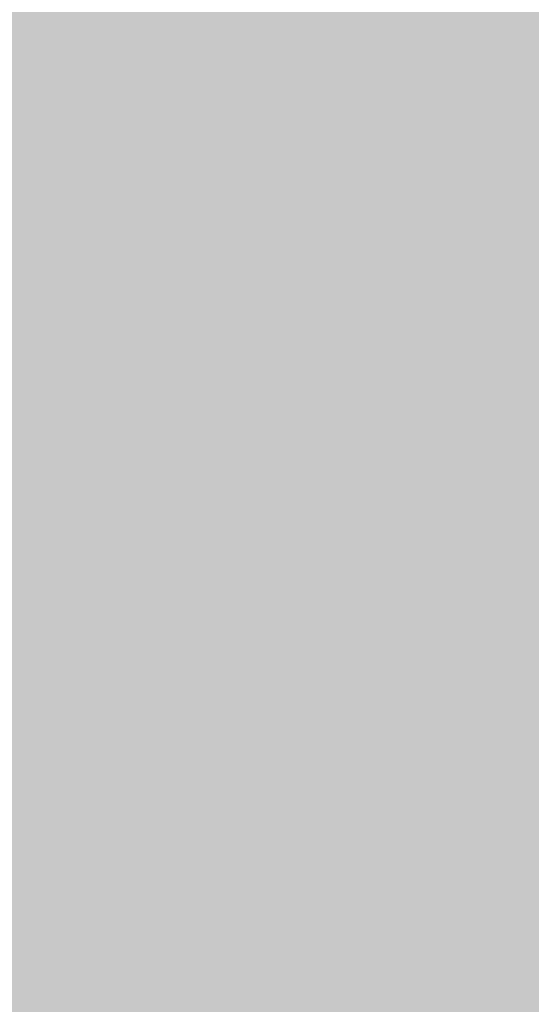
# Model space of a CAD drawing. Units: inches. Extents: x 2083 to 3317, y 1141 to 2115.
# Tile 226 of 256: x 3123.979 to 3126.132, y 1267.234 to 1271.372. Entities that reach past the tile are written whole.
import ezdxf

# ---------------------------------------------------------------- set-up
doc = ezdxf.new("R2010")
doc.units = ezdxf.units.IN
doc.layers.add('A-ANNO-DIMS', color=2, linetype='Continuous', lineweight=18)
doc.layers.add('A-WALL-PATT', color=251, linetype='Continuous', lineweight=13, true_color=0x636466)
doc.styles.get("Standard").update_dxf_attribs({"font": 'arial.ttf'})
doc.dimstyles.new('ISO-25', dxfattribs={"dimtxt": 12, "dimasz": 12, "dimexe": 1.25, "dimexo": 0.625, "dimtad": 1, "dimlunit": 3, "dimtxsty": 'Standard', "dimcen": 2.5, "dimadec": 0, "dimazin": 0, "dimtfac": 1, "dimtmove": 0, "dimatfit": 3, "dimfxl": 1, "dimarcsym": 0})

# ---------------------------------------------------------------- blocks, each defined once
blk = doc.blocks.new('*D26')
at = {"layer": 'A-ANNO-DIMS', "color": 0, "lineweight": -2, "transparency": 16777216}
for p, q in [((3088.9858, 1274.9151), (3088.9858, 1270.952)), ((3111.24, 1274.9151), (3111.24, 1270.952)), ((3076.9858, 1272.202), (2840.2624, 1272.202)), ((3111.24, 1272.202), (3088.9858, 1272.202)), ((3123.24, 1272.202), (3135.24, 1272.202))]:
    blk.add_line(p, q, dxfattribs=at)
at = {"layer": 'A-ANNO-DIMS', "color": 0, "transparency": 16777216}
for points in [[(3076.9858, 1274.202), (3076.9858, 1270.202), (3088.9858, 1272.202)], [(3123.24, 1274.202), (3123.24, 1270.202), (3111.24, 1272.202)]]:
    blk.add_solid(points, dxfattribs=at)
at = {"layer": 'Defpoints', "color": 0, "transparency": 16777216}
for p in [(3088.9858, 1275.5401), (3111.24, 1275.5401), (3088.9858, 1272.202)]:
    blk.add_point(p, dxfattribs=at)
at = {"layer": 'A-ANNO-DIMS', "color": 0, "transparency": 16777216, "insert": (2952.6241, 1279.0316), "char_height": 12, "attachment_point": 5}
blk.add_mtext('NIGHTSTAND 1\'-10 1/2" TYP.', dxfattribs=at)
blk = doc.blocks.new('*D27')
at = {"layer": 'A-ANNO-DIMS', "color": 0, "lineweight": -2, "transparency": 16777216}
for p, q in [((3114.5782, 1309.7943), (3114.5782, 1321.7943)), ((3111.865, 1297.7943), (3115.8282, 1297.7943)), ((3114.5782, 1297.7943), (3114.5782, 1275.5401)), ((3111.865, 1275.5401), (3115.8282, 1275.5401)), ((3114.5782, 1263.5401), (3114.5782, 1140.9886))]:
    blk.add_line(p, q, dxfattribs=at)
at = {"layer": 'A-ANNO-DIMS', "color": 0, "transparency": 16777216}
for points in [[(3112.5782, 1309.7943), (3116.5782, 1309.7943), (3114.5782, 1297.7943)], [(3112.5782, 1263.5401), (3116.5782, 1263.5401), (3114.5782, 1275.5401)]]:
    blk.add_solid(points, dxfattribs=at)
at = {"layer": 'Defpoints', "color": 0, "transparency": 16777216}
for p in [(3111.24, 1297.7943), (3111.24, 1275.5401), (3114.5782, 1275.5401)]:
    blk.add_point(p, dxfattribs=at)
at = {"layer": 'A-ANNO-DIMS', "color": 0, "transparency": 16777216, "insert": (3107.7485, 1196.2643), "char_height": 12, "attachment_point": 5, "rotation": 90}
blk.add_mtext('1\'-10 1/2" TYP.', dxfattribs=at)

msp = doc.modelspace()

# ---------------------------------------------------------------- hatches: boundary and pattern name
at = {"layer": 'A-WALL-PATT'}
h = msp.add_hatch(color=256, dxfattribs=at)
h.dxf.hatch_style = 1
h.paths.add_polyline_path([(3126.9598, 2020.7614), (2748.9598, 2020.7614), (2604.9598, 2020.7614), (2226.9598, 2020.7614), (2226.9598, 1702.7614), (2466.9598, 1702.7614), (2466.9598, 1582.7614), (2418.9598, 1582.7614), (2418.9598, 1477.7614), (2226.9598, 1477.7614), (2226.9598, 1263.2614), (2544.9598, 1263.2614), (2544.9598, 1411.7614), (2604.9598, 1411.7614), (2685.9598, 1411.7614), (2685.9598, 1420.7614), (2604.9598, 1420.7614), (2604.9598, 1573.7614), (2604.9598, 1702.7614), (2604.9598, 2011.7614), (2748.9598, 2011.7614), (2748.9598, 1702.7614), (2862.9598, 1702.7614), (2862.9598, 1621.7614), (2871.9598, 1621.7614), (2871.9598, 1702.7614), (2883.9598, 1702.7614), (2883.9598, 1706.9395, -0.026459), (2883.9598, 1711.7614), (2757.9598, 1711.7614), (2757.9598, 1807.7614), (2787.9598, 1807.7614), (2787.9598, 1812.2614), (2757.9598, 1812.2614), (2757.9598, 2011.7614), (2877.9598, 2011.7614), (2877.9598, 1812.2614), (2847.9598, 1812.2614), (2847.9598, 1807.7614), (2889.8357, 1807.7614), (2889.8357, 1812.2614), (2882.4598, 1812.2614), (2882.4598, 2011.7614), (3117.9598, 2011.7614), (3117.9598, 1812.2614), (2937.8357, 1812.2614), (2937.8357, 1807.7614), (2995.7098, 1807.7614), (2995.7098, 1796.1177), (3000.2098, 1796.1177), (3000.2098, 1807.7614), (3117.9598, 1807.7614), (3117.9598, 1711.7614), (3000.2098, 1711.7614), (3000.2098, 1760.1177), (2998.5727, 1760.1177, -0.020711), (2995.7098, 1760.1177), (2995.7098, 1711.7614), (2931.9598, 1711.7614), (2931.9598, 1702.7614), (3126.9598, 1702.7614)])
h.paths.add_polyline_path([(2471.4598, 2011.7614), (2471.4598, 1810.0114), (2462.7169, 1810.0114), (2462.7169, 1805.5114), (2505.9598, 1805.5114), (2505.9598, 1810.0114), (2475.9598, 1810.0114), (2475.9598, 2011.7614), (2595.9598, 2011.7614), (2595.9598, 1810.0114), (2565.9598, 1810.0114), (2565.9598, 1805.5114), (2595.9598, 1805.5114), (2595.9598, 1711.7614), (2235.9598, 1711.7614), (2235.9598, 1805.5114), (2353.7098, 1805.5114), (2353.7098, 1796.0542), (2358.2098, 1796.0542), (2358.2098, 1805.5114), (2414.7169, 1805.5114), (2414.7169, 1810.0114), (2235.9598, 1810.0114), (2235.9598, 2011.7614)], flags=16)
h.paths.add_polyline_path([(2270.2047, 1994.61), (2270.2047, 1970.61), (2246.2047, 1970.61), (2246.2047, 1994.61)], flags=0)
edge = h.paths.add_edge_path(flags=0)
edge.add_ellipse((2332.0274, 1899.7982), major_axis=(-3.043, 3.043), ratio=0.168252, start_angle=-161.3322, end_angle=-156.3071, ccw=False)
edge.add_ellipse((2333.082, 1898.7435), major_axis=(-1.0546, 1.0546), ratio=0.453532, start_angle=-123.371, end_angle=-94.1591)
edge = h.paths.add_edge_path(flags=0)
edge.add_ellipse((2332.0274, 1968.8763), major_axis=(3.043, 3.043), ratio=0.168252, start_angle=18.6678, end_angle=23.6929)
edge.add_spline(control_points=[(2332.9256, 1970.6911), (2332.2268, 1970.3361), (2330.8937, 1969.6589), (2328.4131, 1970.9321), (2327.2039, 1967.7487), (2324.7096, 1969.9556), (2322.5328, 1967.0124), (2320.0128, 1971.2958), (2317.6803, 1968.1578), (2316.0405, 1967.102), (2315.4269, 1966.8096)], knot_values=[0, 0, 0, 0, 2.267059, 4.324559, 6.685584, 8.878641, 11.121502, 14.300359, 17.755284, 19.732645, 19.732645, 19.732645, 19.732645], degree=3, periodic=0)
edge.add_ellipse((2332.0274, 1968.8763), major_axis=(3.043, 3.043), ratio=0.168252, start_angle=18.6678, end_angle=23.6929, ccw=False)
edge.add_ellipse((2333.082, 1969.9309), major_axis=(1.0546, 1.0546), ratio=0.453532, start_angle=56.629, end_angle=85.8409, ccw=False)
edge = h.paths.add_edge_path(flags=0)
edge.add_spline(control_points=[(2296.4283, 1967.9879), (2293.6278, 1965.3363), (2287.7036, 1959.7271), (2299.7439, 1949.9957), (2294.5326, 1935.6685), (2290.5732, 1920.6035), (2293.3941, 1909.9737), (2296.1854, 1904.9665)], knot_values=[0.099185, 0.099185, 0.099185, 0.099185, 0.345301, 0.619822, 0.982653, 1.386093, 1.810555, 1.810555, 1.810555, 1.810555], degree=3, periodic=0)
edge.add_spline(control_points=[(2296.1854, 1904.9665), (2297.3836, 1902.6193), (2298.001, 1901.9493), (2298.553, 1901.4682)], knot_values=[0.006246, 0.006246, 0.006246, 0.006246, 0.055476, 0.055476, 0.055476, 0.055476], degree=3, periodic=0)
edge.add_spline(control_points=[(2298.553, 1901.4682), (2297.2586, 1900.9232), (2295.2253, 1900.2321), (2293.0602, 1900.6142), (2292.1014, 1900.7884), (2292.0896, 1900.7906)], knot_values=[0.312835, 0.312835, 0.312835, 0.312835, 0.40178, 0.474987, 0.475903, 0.475903, 0.475903, 0.475903], degree=3, periodic=0)
edge.add_arc((2292.7936, 1904.6641), 3.937, 215.4209, 259.6982, ccw=False)
edge.add_spline(control_points=[(2289.5853, 1902.3823), (2289.4767, 1902.5351), (2289.3685, 1902.688), (2289.2609, 1902.8412)], knot_values=[0.102872, 0.102872, 0.102872, 0.102872, 0.116896, 0.116896, 0.116896, 0.116896], degree=3, periodic=0)
edge.add_spline(control_points=[(2289.2609, 1902.8412), (2288.6866, 1902.5502), (2287.64, 1902.0199), (2285.8813, 1901.874), (2283.853, 1901.5044), (2281.72, 1899.7105), (2278.467, 1899.4929), (2276.1571, 1901.8832), (2272.259, 1899.8041), (2267.7776, 1901.8432), (2262.2439, 1900.184), (2257.4149, 1901.7821), (2254.3184, 1900.7261), (2253.1783, 1900.3373)], knot_values=[0, 0, 0, 0, 1.907977, 3.477176, 5.261074, 7.972851, 11.680248, 13.717921, 16.939592, 22.789562, 27.502503, 33.595215, 37.145618, 37.145618, 37.145618, 37.145618], degree=3, periodic=0)
edge.add_line((2253.1783, 1900.3373), (2250.2442, 1902.8412))
edge.add_line((2250.2442, 1902.8412), (2250.2442, 1965.8333))
edge.add_line((2250.2442, 1965.8333), (2253.1783, 1968.3371))
edge.add_spline(control_points=[(2253.1783, 1968.3371), (2254.3184, 1967.9483), (2257.4149, 1966.8924), (2262.2439, 1968.4904), (2267.7776, 1966.8313), (2271.5267, 1968.5372), (2273.8759, 1967.8283), (2274.2067, 1967.7276)], knot_values=[0, 0, 0, 0, 0.09018, 0.244935, 0.364644, 0.513233, 0.537855, 0.537855, 0.537855, 0.537855], degree=3, periodic=0)
edge.add_arc((2274.3529, 1963.7933), 3.937, 72.0511, 92.1279, ccw=False)
edge.add_arc((2281.2969, 1985.23), 18.5963, 252.05113, 288.56572)
edge.add_arc((2292.3167, 1956.0289), 12.6461, 71.02679, 113.77822, ccw=False)
edge = h.paths.add_edge_path(flags=0)
edge.add_spline(control_points=[(2274.8994, 1951.8562), (2275.0662, 1951.6166), (2275.2327, 1951.3766), (2275.398, 1951.1359)], knot_values=[1.409916, 1.409916, 1.409916, 1.409916, 1.43159, 1.43159, 1.43159, 1.43159], degree=3, periodic=0)
edge.add_spline(control_points=[(2275.398, 1951.1359), (2275.7921, 1950.5619), (2276.1792, 1949.9838), (2276.5455, 1949.3971)], knot_values=[1.358238, 1.358238, 1.358238, 1.358238, 1.409916, 1.409916, 1.409916, 1.409916], degree=3, periodic=0)
edge.add_line((2276.5455, 1949.3971), (2277.4373, 1947.8622))
edge.add_spline(control_points=[(2277.4373, 1947.8622), (2276.3038, 1945.6731), (2274.6397, 1942.4269), (2274.6316, 1938.0939), (2272.7991, 1930.8515), (2274.3564, 1943.897), (2275.9477, 1947.9234), (2276.5455, 1949.3971)], knot_values=[0.005632, 0.005632, 0.005632, 0.005632, 0.186014, 0.266002, 0.357087, 0.59639, 0.739732, 0.739732, 0.739732, 0.739732], degree=3, periodic=0)
edge.add_spline(control_points=[(2276.5455, 1949.3971), (2276.1792, 1949.9838), (2275.7921, 1950.5619), (2275.398, 1951.1359)], knot_values=[1.358238, 1.358238, 1.358238, 1.358238, 1.409916, 1.409916, 1.409916, 1.409916], degree=3, periodic=0)
edge.add_spline(control_points=[(2275.398, 1951.1359), (2274.9425, 1950.0805), (2274.2078, 1948.0253), (2273.9346, 1944.8515), (2272.4685, 1937.6275), (2273.4662, 1945.6965), (2274.7006, 1951.0595), (2274.8994, 1951.8562)], knot_values=[0.104364, 0.104364, 0.104364, 0.104364, 0.189636, 0.269624, 0.36071, 0.600013, 0.644622, 0.644622, 0.644622, 0.644622], degree=3, periodic=0)
h.paths.add_polyline_path([(2269.1675, 1963.1276, -0.357527), (2268.1706, 1960.9764, -0.092561), (2268.1706, 1939.4363, -0.357527), (2269.1675, 1937.2851, -0.357527), (2267.0163, 1938.282, -0.164785), (2254.6856, 1938.282, -0.357527), (2252.5344, 1937.2851, -0.357527), (2253.5313, 1939.4363, -0.092561), (2253.5313, 1960.9764, -0.357527), (2252.5344, 1963.1276, -0.357527), (2254.6856, 1962.1307, -0.164785), (2267.0163, 1962.1307, -0.357527)], flags=0)
h.paths.add_polyline_path([(2248.8741, 1967.8018), (2248.8741, 1957.0277), (2249.4578, 1957.0277), (2249.4578, 1911.6468), (2248.8741, 1911.6468), (2248.8741, 1900.8727), (2246.5119, 1900.8727, 0.197327), (2244.1497, 1902.4569), (2244.1497, 1966.2176, 0.197327), (2246.5119, 1967.8018)], flags=0)
h.paths.add_polyline_path([(2269.1675, 1931.3893, -0.357527), (2268.1706, 1929.2381, -0.092561), (2268.1706, 1907.6981, -0.357527), (2269.1675, 1905.5469, -0.357527), (2267.0163, 1906.5438, -0.164785), (2254.6856, 1906.5438, -0.357527), (2252.5344, 1905.5469, -0.357527), (2253.5313, 1907.6981, -0.092561), (2253.5313, 1929.2381, -0.357527), (2252.5344, 1931.3893, -0.357527), (2254.6856, 1930.3925, -0.164785), (2267.0163, 1930.3925, -0.357527)], flags=0)
edge = h.paths.add_edge_path(flags=0)
edge.add_spline(control_points=[(2276.1969, 1906.7237), (2276.1681, 1909.0289), (2276.114, 1913.3719), (2270.5984, 1924.925), (2273.9052, 1919.0128), (2275.9217, 1916.2621), (2275.4746, 1912.4021), (2277.2579, 1910.3806), (2276.696, 1908.225), (2276.6462, 1906.813), (2276.6178, 1906.0084)], knot_values=[0, 0, 0, 0, 8.61026, 16.221274, 18.843057, 23.804898, 27.440828, 29.356102, 31.203478, 33.650687, 33.650687, 33.650687, 33.650687], degree=3, periodic=0)
edge.add_spline(control_points=[(2276.6178, 1906.0084), (2276.6233, 1905.6241), (2276.4977, 1904.6287), (2275.4418, 1903.8547), (2274.9373, 1903.0804), (2274.8591, 1902.8412)], knot_values=[0.156488, 0.156488, 0.156488, 0.156488, 0.184398, 0.231376, 0.250598, 0.250598, 0.250598, 0.250598], degree=3, periodic=0)
edge.add_line((2274.8591, 1902.8412), (2276.506, 1902.8412))
edge.add_spline(control_points=[(2276.506, 1902.8412), (2276.7883, 1903.0849), (2277.6651, 1904.1252), (2278.2495, 1904.3407), (2277.6539, 1908.5274), (2278.1557, 1906.2278), (2278.1005, 1905.2859), (2278.8467, 1904.069), (2277.8568, 1903.4149), (2277.8742, 1902.991), (2277.9036, 1902.8412)], knot_values=[0.059574, 0.059574, 0.059574, 0.059574, 0.080753, 0.103741, 0.16972, 0.176036, 0.207137, 0.240474, 0.262341, 0.27366, 0.27366, 0.27366, 0.27366], degree=3, periodic=0)
edge.add_line((2277.9036, 1902.8412), (2280.0298, 1902.8412))
edge.add_spline(control_points=[(2280.0298, 1902.8412), (2279.8882, 1903.0884), (2279.4993, 1903.9816), (2280.1523, 1905.9393), (2278.1036, 1909.6578), (2279.7624, 1907.1853), (2280.3279, 1904.8749), (2280.4851, 1903.4896), (2281.4633, 1903.2494), (2281.7583, 1902.9365), (2281.834, 1902.8412)], knot_values=[0.013856, 0.013856, 0.013856, 0.013856, 0.034874, 0.088867, 0.107879, 0.126738, 0.158714, 0.193757, 0.217487, 0.226722, 0.226722, 0.226722, 0.226722], degree=3, periodic=0)
edge.add_spline(control_points=[(2281.834, 1902.8412), (2281.7875, 1902.8267), (2281.647, 1902.783), (2281.3955, 1902.8595), (2281.0881, 1902.9852), (2280.7207, 1903.0609), (2280.3335, 1903.0257), (2280.1248, 1902.8989), (2280.0298, 1902.8412)], knot_values=[0, 0, 0, 0, 0.14413, 0.435517, 0.749276, 1.153046, 1.548371, 1.878348, 1.878348, 1.878348, 1.878348], degree=3, periodic=0)
edge.add_line((2280.0298, 1902.8412), (2277.9036, 1902.8412))
edge.add_spline(control_points=[(2277.9036, 1902.8412), (2277.8929, 1902.7959), (2277.8654, 1902.6796), (2277.6075, 1902.6875), (2277.2741, 1902.8007), (2276.8379, 1902.6198), (2276.5838, 1902.7893), (2276.506, 1902.8412)], knot_values=[0, 0, 0, 0, 0.127189, 0.326199, 0.628009, 1.24357, 1.515331, 1.515331, 1.515331, 1.515331], degree=3, periodic=0)
edge.add_line((2276.506, 1902.8412), (2274.8591, 1902.8412))
edge.add_spline(control_points=[(2274.8591, 1902.8412), (2274.8144, 1902.8986), (2274.7251, 1903.0134), (2274.4935, 1903.119), (2274.2443, 1902.9605), (2273.9371, 1903.1849), (2273.614, 1902.9831), (2273.4083, 1902.883), (2273.3223, 1902.8412)], knot_values=[0, 0, 0, 0, 0.21843, 0.436957, 0.687977, 0.990379, 1.398396, 1.69185, 1.69185, 1.69185, 1.69185], degree=3, periodic=0)
edge.add_spline(control_points=[(2273.3223, 1902.8412), (2273.6167, 1903.4457), (2274.274, 1904.5383), (2276.0272, 1904.5737), (2276.207, 1906.5836), (2276.1969, 1906.7237)], knot_values=[0.012227, 0.012227, 0.012227, 0.012227, 0.059472, 0.106218, 0.134458, 0.134458, 0.134458, 0.134458], degree=3, periodic=0)
h.paths.add_polyline_path([(2270.7761, 1897.7898), (2270.7761, 1873.7898), (2246.7761, 1873.7898), (2246.7761, 1897.7898)], flags=0)
h.paths.add_polyline_path([(2353.7098, 1760.0051), (2353.7098, 1760.0542), (2358.2098, 1760.0542, -0.033729)], flags=0)
h.paths.add_polyline_path([(2321.8191, 1737.5292), (2341.9953, 1737.5292, -0.414214), (2343.2033, 1736.3212), (2343.2033, 1721.0206, -0.414214), (2341.9953, 1719.8127), (2321.8191, 1719.8127, -0.414214), (2320.6112, 1721.0206), (2320.6112, 1736.3212, -0.414214)], flags=0)
h.paths.add_polyline_path([(2324.235, 1736.3212), (2339.5794, 1736.3212, -0.414214), (2341.9953, 1733.9053), (2341.9953, 1725.4497, -0.414214), (2339.5794, 1723.0338), (2333.6806, 1723.0338), (2333.8453, 1722.0455, -0.870646), (2335.4254, 1721.8259, -0.767327), (2333.9227, 1721.4232), (2331.291, 1721.4232, -0.767327), (2329.7883, 1721.8259, -0.870646), (2331.3684, 1722.0455), (2331.5331, 1723.0338), (2324.235, 1723.0338, -0.414214), (2321.8191, 1725.4497), (2321.8191, 1733.9053, -0.414214)], flags=0)
h.paths.add_polyline_path([(2570.4838, 1928.6154), (2589.6838, 1928.6154), (2590.1688, 1928.6154), (2590.1688, 1904.9934), (2570.4838, 1904.9934)], flags=0)
h.paths.add_polyline_path([(2574.4473, 1927.2638, -1), (2572.8288, 1927.2638, -1)], flags=0)
h.paths.add_polyline_path([(2573.0899, 1926.9409), (2573.925, 1927.776), (2574.1477, 1927.5533), (2573.3126, 1926.7182)], flags=0)
h.paths.add_polyline_path([(2578.7791, 1919.7296, -1), (2571.5917, 1919.7296, -1)], flags=0)
h.paths.add_polyline_path([(2578.3854, 1919.7296, -1), (2571.9854, 1919.7296, -1)], flags=0)
h.paths.add_polyline_path([(2331.5958, 1729.4762, -1), (2333.618, 1729.4762, -1)], flags=0)
h.paths.add_polyline_path([(2578.0342, 1927.2638, -1), (2576.4157, 1927.2638, -1)], flags=0)
h.paths.add_polyline_path([(2576.6889, 1927.5311), (2576.9116, 1927.7538), (2577.7467, 1926.9186), (2577.524, 1926.6959)], flags=0)
h.paths.add_polyline_path([(2578.1391, 1909.8595, -1), (2572.2317, 1909.8595, -1)], flags=0)
h.paths.add_polyline_path([(2577.7454, 1909.8595, -1), (2572.6254, 1909.8595, -1)], flags=0)
h.paths.add_polyline_path([(2583.7977, 1927.2638, -1), (2582.1792, 1927.2638, -1)], flags=0)
h.paths.add_polyline_path([(2582.7186, 1927.7538), (2583.5538, 1926.9186), (2583.3311, 1926.6959), (2582.4959, 1927.5311)], flags=0)
h.paths.add_polyline_path([(2582.4959, 1927.5311), (2582.7186, 1927.7538), (2583.5538, 1926.9186), (2583.3311, 1926.6959)], flags=0)
h.paths.add_polyline_path([(2587.7391, 1920.5296, -1), (2581.8317, 1920.5296, -1)], flags=0)
h.paths.add_polyline_path([(2587.3454, 1920.5296, -1), (2582.2254, 1920.5296, -1)], flags=0)
h.paths.add_polyline_path([(2587.3846, 1927.2638, -1), (2585.7661, 1927.2638, -1)], flags=0)
h.paths.add_polyline_path([(2586.082, 1926.9802), (2586.9172, 1927.8154), (2587.1399, 1927.5927), (2586.3047, 1926.7575)], flags=0)
h.paths.add_polyline_path([(2588.3791, 1910.6595, -1), (2581.1917, 1910.6595, -1)], flags=0)
h.paths.add_polyline_path([(2587.9854, 1910.6595, -1), (2581.5854, 1910.6595, -1)], flags=0)
h.paths.add_polyline_path([(2417.1677, 1729.4779), (2437.3439, 1729.4779, -0.414214), (2438.5519, 1728.2699), (2438.5519, 1712.9693, -0.414214), (2437.3439, 1711.7614), (2417.1677, 1711.7614, -0.414214), (2415.9598, 1712.9693), (2415.9598, 1728.2699, -0.414214)], flags=0)
h.paths.add_polyline_path([(2419.5836, 1728.2699), (2434.928, 1728.2699, -0.414214), (2437.3439, 1725.8541), (2437.3439, 1717.3984, -0.414214), (2434.928, 1714.9825), (2429.0292, 1714.9825), (2429.1939, 1713.9942, -0.870646), (2430.774, 1713.7746, -0.767327), (2429.2713, 1713.372), (2426.6396, 1713.372, -0.767327), (2425.1369, 1713.7746, -0.870646), (2426.717, 1713.9942), (2426.8817, 1714.9825), (2419.5836, 1714.9825, -0.414214), (2417.1677, 1717.3984), (2417.1677, 1725.8541, -0.414214)], flags=0)
h.paths.add_polyline_path([(2419.5836, 1728.2699), (2434.928, 1728.2699, -0.414214), (2437.3439, 1725.8541), (2437.3439, 1717.3984, -0.414214), (2434.928, 1714.9825), (2429.0292, 1714.9825), (2428.3581, 1719.009), (2427.5528, 1719.009), (2426.8817, 1714.9825), (2419.5836, 1714.9825, -0.414214), (2417.1677, 1717.3984), (2417.1677, 1725.8541, -0.414214)], flags=0)
h.paths.add_polyline_path([(2426.9444, 1721.4249, -1), (2428.9666, 1721.4249, -1)], flags=0)
h.paths.add_polyline_path([(2475.9598, 1702.7614), (2595.9598, 1702.7614), (2595.9598, 1582.7614), (2475.9598, 1582.7614)], flags=16)
h.paths.add_polyline_path([(2427.9598, 1573.7614), (2595.9598, 1573.7614), (2595.9598, 1468.7614), (2595.9598, 1420.7614), (2384.4598, 1420.7614), (2384.4598, 1468.7614), (2427.9598, 1468.7614)], flags=16)
h.paths.add_polyline_path([(2379.9598, 1468.7614), (2379.9598, 1420.7614), (2235.9598, 1420.7614), (2235.9598, 1468.7614)], flags=16)
h.paths.add_polyline_path([(2317.816, 1466.6958), (2337.9922, 1466.6958, -0.414214), (2339.2002, 1465.4878), (2339.2002, 1450.1872, -0.414214), (2337.9922, 1448.9792), (2317.816, 1448.9792, -0.414214), (2316.6081, 1450.1872), (2316.6081, 1465.4878, -0.414214)], flags=0)
h.paths.add_polyline_path([(2320.2319, 1465.4878), (2335.5763, 1465.4878, -0.414214), (2337.9922, 1463.0719), (2337.9922, 1454.6163, -0.414214), (2335.5763, 1452.2004), (2329.6775, 1452.2004), (2329.8422, 1451.212, -0.870646), (2331.4223, 1450.9925, -0.767327), (2329.9196, 1450.5898), (2327.2879, 1450.5898, -0.767327), (2325.7852, 1450.9925, -0.870646), (2327.3653, 1451.212), (2327.53, 1452.2004), (2320.2319, 1452.2004, -0.414214), (2317.816, 1454.6163), (2317.816, 1463.0719, -0.414214)], flags=0)
h.paths.add_polyline_path([(2320.2319, 1465.4878), (2335.5763, 1465.4878, -0.414214), (2337.9922, 1463.0719), (2337.9922, 1454.6163, -0.414214), (2335.5763, 1452.2004), (2329.6775, 1452.2004), (2329.0064, 1456.2269), (2328.2011, 1456.2269), (2327.53, 1452.2004), (2320.2319, 1452.2004, -0.414214), (2317.816, 1454.6163), (2317.816, 1463.0719, -0.414214)], flags=0)
h.paths.add_polyline_path([(2327.5926, 1458.6428, -1), (2329.6148, 1458.6428, -1)], flags=0)
h.paths.add_polyline_path([(2244.4117, 1433.3405), (2241.9209, 1433.3405, -0.414214), (2240.0179, 1435.2435), (2240.0179, 1440.9528, -0.414211), (2241.9209, 1442.8559), (2244.4117, 1442.8559, -1.976472)], flags=0)
h.paths.add_polyline_path([(2245.3569, 1434.3975, -0.414214), (2245.3569, 1441.7988, -2.144098)], flags=0)
h.paths.add_polyline_path([(2535.9598, 1416.2614), (2535.9598, 1272.2614), (2235.9598, 1272.2614), (2235.9598, 1416.2614)], flags=16)
h.paths.add_polyline_path([(2260.1196, 1384.2928), (2260.1196, 1362.0386), (2237.8654, 1362.0386), (2237.8654, 1384.2928)], flags=0)
edge = h.paths.add_edge_path(flags=0)
edge.add_line((2318.2518, 1362.0933), (2318.1458, 1362.001))
edge.add_ellipse((2317.4451, 1360.431), major_axis=(2.8216, 2.8216), ratio=0.168252, start_angle=18.6678, end_angle=20.9481, ccw=False)
edge.add_ellipse((2318.423, 1361.409), major_axis=(0.9779, 0.9779), ratio=0.453532, start_angle=56.629, end_angle=70.2262, ccw=False)
edge = h.paths.add_edge_path(flags=0)
edge.add_line((2319.1074, 1295.5711), (2319.015, 1295.6771))
edge.add_ellipse((2317.4451, 1296.3778), major_axis=(-2.8216, 2.8216), ratio=0.168252, start_angle=-161.3322, end_angle=-159.0519, ccw=False)
edge.add_ellipse((2318.423, 1295.3999), major_axis=(-0.9779, 0.9779), ratio=0.453532, start_angle=-123.371, end_angle=-109.7738)
edge = h.paths.add_edge_path(flags=0)
edge.add_spline(control_points=[(2284.2103, 1301.1702), (2284.5807, 1300.4447), (2284.8912, 1299.892), (2285.1596, 1299.461)], knot_values=[0.039066, 0.039066, 0.039066, 0.039066, 0.055476, 0.055476, 0.055476, 0.055476], degree=3, periodic=0)
edge.add_line((2285.1596, 1299.461), (2284.2103, 1301.1702))
edge = h.paths.add_edge_path(flags=0)
edge.add_line((2280.4125, 1297.298), (2283.37, 1297.0361))
edge.add_line((2283.37, 1297.0361), (2286.4057, 1297.9263))
edge.add_spline(control_points=[(2286.4057, 1297.9263), (2285.3055, 1297.4631), (2284.3448, 1297.1292), (2283.37, 1297.0361)], knot_values=[0.394369, 0.394369, 0.394369, 0.394369, 0.475903, 0.475903, 0.475903, 0.475903], degree=3, periodic=0)
edge.add_spline(control_points=[(2283.37, 1297.0361), (2283.2814, 1297.0277), (2282.3163, 1296.9573), (2281.3125, 1297.1345), (2280.4234, 1297.296), (2280.4125, 1297.298)], knot_values=[0.312835, 0.312835, 0.312835, 0.312835, 0.320246, 0.393453, 0.394369, 0.394369, 0.394369, 0.394369], degree=3, periodic=0)
edge = h.paths.add_edge_path(flags=0)
edge.add_line((2284.4356, 1359.6073), (2280.4463, 1355.328))
edge.add_line((2280.4463, 1355.328), (2279.58, 1351.0178))
edge.add_line((2279.58, 1351.0178), (2282.413, 1346.5804))
edge.add_spline(control_points=[(2282.413, 1346.5804), (2283.1533, 1345.5892), (2284.2529, 1344.0289), (2284.801, 1342.3872), (2284.9352, 1341.8055)], knot_values=[1.240098, 1.240098, 1.240098, 1.240098, 1.332892, 1.382712, 1.382712, 1.382712, 1.382712], degree=3, periodic=0)
edge.add_spline(control_points=[(2284.9352, 1341.8055), (2285.3191, 1340.1406), (2285.233, 1338.4092), (2284.9099, 1336.6541)], knot_values=[1.097484, 1.097484, 1.097484, 1.097484, 1.240098, 1.240098, 1.240098, 1.240098], degree=3, periodic=0)
edge.add_spline(control_points=[(2284.9099, 1336.6541), (2284.5868, 1334.899), (2284.0267, 1333.1203), (2283.4626, 1331.3606)], knot_values=[0.95487, 0.95487, 0.95487, 0.95487, 1.097484, 1.097484, 1.097484, 1.097484], degree=3, periodic=0)
edge.add_line((2283.4626, 1331.3606), (2281.8904, 1326.1534))
edge.add_line((2281.8904, 1326.1534), (2280.7563, 1321.0561))
edge.add_line((2280.7563, 1321.0561), (2280.2992, 1316.002))
edge.add_line((2280.2992, 1316.002), (2280.7159, 1310.9501))
edge.add_line((2280.7159, 1310.9501), (2282.0281, 1305.9721))
edge.add_line((2282.0281, 1305.9721), (2284.2103, 1301.1702))
edge.add_spline(control_points=[(2284.2103, 1301.1702), (2283.3407, 1302.7302), (2282.6119, 1304.3365), (2282.0281, 1305.9721)], knot_values=[0.099185, 0.099185, 0.099185, 0.099185, 0.241799, 0.241799, 0.241799, 0.241799], degree=3, periodic=0)
edge.add_spline(control_points=[(2282.0281, 1305.9721), (2281.4443, 1307.6078), (2281.0055, 1309.2728), (2280.7159, 1310.9501)], knot_values=[0.241799, 0.241799, 0.241799, 0.241799, 0.384413, 0.384413, 0.384413, 0.384413], degree=3, periodic=0)
edge.add_spline(control_points=[(2280.7159, 1310.9501), (2280.4332, 1312.5876), (2280.2894, 1314.277), (2280.2989, 1315.962), (2280.2992, 1316.002)], knot_values=[0.384413, 0.384413, 0.384413, 0.384413, 0.523647, 0.527028, 0.527028, 0.527028, 0.527028], degree=3, periodic=0)
edge.add_spline(control_points=[(2280.2992, 1316.002), (2280.3123, 1317.687), (2280.4779, 1319.3679), (2280.7563, 1321.0561)], knot_values=[0.527028, 0.527028, 0.527028, 0.527028, 0.669642, 0.669642, 0.669642, 0.669642], degree=3, periodic=0)
edge.add_spline(control_points=[(2280.7563, 1321.0561), (2281.0346, 1322.7443), (2281.4259, 1324.4396), (2281.8904, 1326.1534)], knot_values=[0.669642, 0.669642, 0.669642, 0.669642, 0.812256, 0.812256, 0.812256, 0.812256], degree=3, periodic=0)
edge.add_spline(control_points=[(2281.8904, 1326.1534), (2282.2644, 1327.5333), (2282.7879, 1329.2618), (2283.3528, 1331.0178), (2283.4626, 1331.3606)], knot_values=[0.812256, 0.812256, 0.812256, 0.812256, 0.927087, 0.95487, 0.95487, 0.95487, 0.95487], degree=3, periodic=0)
edge.add_line((2283.4626, 1331.3606), (2284.9099, 1336.6541))
edge.add_line((2284.9099, 1336.6541), (2284.9352, 1341.8055))
edge.add_line((2284.9352, 1341.8055), (2282.413, 1346.5804))
edge.add_spline(control_points=[(2282.413, 1346.5804), (2281.2751, 1348.1038), (2280.0784, 1349.5703), (2279.58, 1351.0178)], knot_values=[1.382712, 1.382712, 1.382712, 1.382712, 1.525326, 1.525326, 1.525326, 1.525326], degree=3, periodic=0)
edge.add_spline(control_points=[(2279.58, 1351.0178), (2279.4433, 1351.4147), (2279.1363, 1352.8569), (2279.7352, 1354.2904), (2280.4463, 1355.328)], knot_values=[1.525326, 1.525326, 1.525326, 1.525326, 1.564439, 1.667941, 1.667941, 1.667941, 1.667941], degree=3, periodic=0)
edge.add_spline(control_points=[(2280.4463, 1355.328), (2281.4261, 1356.7578), (2282.9308, 1358.1826), (2284.4356, 1359.6073)], knot_values=[1.667941, 1.667941, 1.667941, 1.667941, 1.810555, 1.810555, 1.810555, 1.810555], degree=3, periodic=0)
edge.add_arc((2280.6231, 1348.5182), 11.7262, 71.02679, 113.77822)
edge.add_arc((2270.4049, 1375.5952), 17.2436, 252.05113, 288.56572, ccw=False)
edge.add_arc((2263.966, 1355.7178), 3.6506, 72.0511, 92.1279)
edge.add_arc((2263.966, 1355.7178), 3.6506, 92.1279, 177.9851)
edge.add_spline(control_points=[(2260.3176, 1355.8462), (2260.2604, 1354.2207), (2260.5513, 1350.1865), (2262.9993, 1346.7663), (2264.4727, 1344.649)], knot_values=[1.43159, 1.43159, 1.43159, 1.43159, 1.564144, 1.770695, 1.770695, 1.770695, 1.770695], degree=3, periodic=0)
edge.add_line((2264.4727, 1344.649), (2264.9356, 1343.9825))
edge.add_spline(control_points=[(2263.801, 1340.2481), (2263.8432, 1340.5141), (2264.0672, 1341.7565), (2264.5127, 1343.0025), (2264.935, 1343.9811)], knot_values=[0.53657, 0.53657, 0.53657, 0.53657, 0.559349, 0.644622, 0.644622, 0.644622, 0.644622], degree=3, periodic=0)
edge.add_spline(control_points=[(2264.935, 1343.9811), (2265.1178, 1343.715), (2265.2989, 1343.4479), (2265.4768, 1343.1794)], knot_values=[1.384077, 1.384077, 1.384077, 1.384077, 1.409916, 1.409916, 1.409916, 1.409916], degree=3, periodic=0)
edge.add_spline(control_points=[(2265.4768, 1343.1794), (2265.6546, 1342.9108), (2265.8293, 1342.6408), (2265.9991, 1342.3688)], knot_values=[1.358238, 1.358238, 1.358238, 1.358238, 1.384077, 1.384077, 1.384077, 1.384077], degree=3, periodic=0)
edge.add_line((2265.9991, 1342.3688), (2266.826, 1340.9455))
edge.add_spline(control_points=[(2266.826, 1340.9455), (2268.8944, 1337.0897), (2271.3982, 1325.843), (2270.5162, 1310.5686), (2275.9194, 1301.8606), (2277.7895, 1299.1994)], knot_values=[0.116896, 0.116896, 0.116896, 0.116896, 0.472987, 1.050969, 1.313793, 1.313793, 1.313793, 1.313793], degree=3, periodic=0)
edge.add_spline(control_points=[(2277.7895, 1299.1994), (2277.8394, 1299.1285), (2277.8894, 1299.0575), (2277.9396, 1298.9866)], knot_values=[0.109884, 0.109884, 0.109884, 0.109884, 0.116896, 0.116896, 0.116896, 0.116896], degree=3, periodic=0)
edge.add_line((2277.9396, 1298.9866), (2277.7888, 1299.1991))
edge.add_spline(control_points=[(2277.7888, 1299.1991), (2277.2566, 1298.9294), (2276.2864, 1298.4379), (2275.0394, 1298.3344), (2274.3833, 1298.2389), (2274.2153, 1298.2093)], knot_values=[33.12187, 33.12187, 33.12187, 33.12187, 35.029056, 36.598255, 37.144827, 37.144827, 37.144827, 37.144827], degree=3, periodic=0)
edge.add_line((2274.2153, 1298.2093), (2273.0731, 1297.893))
edge.add_spline(control_points=[(2273.0731, 1297.893), (2272.3229, 1297.5798), (2271.0392, 1296.5105), (2269.2484, 1296.2261), (2268.4231, 1296.3747)], knot_values=[26.532584, 26.532584, 26.532584, 26.532584, 29.198919, 31.839101, 31.839101, 31.839101, 31.839101], degree=3, periodic=0)
edge.add_line((2268.4231, 1296.3747), (2263.8785, 1297.4575))
edge.add_spline(control_points=[(2263.8785, 1297.4575), (2263.5561, 1297.3594), (2261.8603, 1296.8387), (2260.2388, 1297.2824), (2258.9335, 1297.5165)], knot_values=[15.919551, 15.919551, 15.919551, 15.919551, 16.939592, 21.226067, 21.226067, 21.226067, 21.226067], degree=3, periodic=0)
edge.add_line((2258.9335, 1297.5165), (2254.0552, 1297.329))
edge.add_spline(control_points=[(2254.0552, 1297.329), (2253.7555, 1297.2958), (2252.1137, 1297.1652), (2250.4619, 1297.5442), (2249.1297, 1297.6679)], knot_values=[5.306517, 5.306517, 5.306517, 5.306517, 6.276435, 10.613034, 10.613034, 10.613034, 10.613034], degree=3, periodic=0)
edge.add_line((2249.1297, 1297.6679), (2244.3316, 1296.8778))
edge.add_line((2244.3316, 1296.8778), (2241.611, 1299.1994))
edge.add_line((2241.611, 1299.1994), (2241.611, 1357.6094))
edge.add_line((2241.611, 1357.6094), (2244.3316, 1359.9311))
edge.add_line((2244.3316, 1359.9311), (2252.7288, 1359.5427))
edge.add_spline(control_points=[(2252.7288, 1359.5427), (2252.8709, 1359.5464), (2253.3057, 1359.5482), (2253.7398, 1359.5143), (2254.0317, 1359.4824)], knot_values=[0.233291, 0.233291, 0.233291, 0.233291, 0.244935, 0.268927, 0.268927, 0.268927, 0.268927], degree=3, periodic=0)
edge.add_line((2254.0317, 1359.4824), (2259.5872, 1359.4164))
edge.add_spline(control_points=[(2259.5872, 1359.4164), (2260.6771, 1359.6285), (2262.0732, 1359.897), (2263.5237, 1359.4593), (2263.8304, 1359.366)], knot_values=[0.422516, 0.422516, 0.422516, 0.422516, 0.513233, 0.537855, 0.537855, 0.537855, 0.537855], degree=3, periodic=0)
edge.add_arc((2263.966, 1355.7178), 3.6506, 72.0511, 92.1279, ccw=False)
edge.add_arc((2270.4049, 1375.5952), 17.2436, 252.05113, 288.56572)
edge.add_arc((2280.6231, 1348.5182), 11.7262, 71.02679, 113.77822, ccw=False)
h.paths.add_polyline_path([(2240.3405, 1359.4347), (2240.3405, 1349.4444), (2240.8818, 1349.4444), (2240.8818, 1307.3645), (2240.3405, 1307.3645), (2240.3405, 1297.3741), (2238.1502, 1297.3741, 0.197327), (2235.9598, 1298.8431), (2235.9598, 1357.9657, 0.197327), (2238.1502, 1359.4347)], flags=0)
h.paths.add_polyline_path([(2259.1578, 1355.1005, -0.357527), (2258.2334, 1353.1058, -0.092561), (2258.2334, 1333.1326, -0.357527), (2259.1578, 1331.1379, -0.357527), (2257.1631, 1332.0622, -0.164785), (2245.7293, 1332.0622, -0.357527), (2243.7346, 1331.1379, -0.357527), (2244.6589, 1333.1326, -0.092561), (2244.6589, 1353.1058, -0.357527), (2243.7346, 1355.1005, -0.357527), (2245.7293, 1354.1761, -0.164785), (2257.1631, 1354.1761, -0.357527)], flags=0)
edge = h.paths.add_edge_path(flags=0)
edge.add_line((2265.9991, 1342.3688), (2266.826, 1340.9455))
edge.add_line((2266.826, 1340.9455), (2265.3076, 1337.8141))
edge.add_line((2265.3076, 1337.8141), (2264.3582, 1334.6529))
edge.add_line((2264.3582, 1334.6529), (2264.262, 1333.7997))
edge.add_spline(control_points=[(2264.262, 1333.7997), (2264.2084, 1333.1871), (2264.1621, 1332.3655), (2264.0071, 1331.4139), (2263.969, 1331.2018)], knot_values=[0.464444, 0.464444, 0.464444, 0.464444, 0.516691, 0.531608, 0.531608, 0.531608, 0.531608], degree=3, periodic=0)
edge.add_spline(control_points=[(2263.969, 1331.2018), (2263.7745, 1330.1189), (2263.4244, 1328.7908), (2263.2574, 1328.5307), (2263.234, 1328.5146)], knot_values=[0.372682, 0.372682, 0.372682, 0.372682, 0.44885, 0.464444, 0.464444, 0.464444, 0.464444], degree=3, periodic=0)
edge.add_spline(control_points=[(2263.234, 1328.5146), (2263.0964, 1328.4202), (2263.1312, 1329.3015), (2263.275, 1330.6157)], knot_values=[0.280919, 0.280919, 0.280919, 0.280919, 0.372682, 0.372682, 0.372682, 0.372682], degree=3, periodic=0)
edge.add_spline(control_points=[(2263.275, 1330.6157), (2263.4187, 1331.93), (2263.6715, 1333.6773), (2263.9699, 1335.315)], knot_values=[0.189157, 0.189157, 0.189157, 0.189157, 0.280919, 0.280919, 0.280919, 0.280919], degree=3, periodic=0)
edge.add_spline(control_points=[(2263.9699, 1335.315), (2264.1005, 1336.0322), (2264.4188, 1337.6219), (2264.7548, 1338.8644), (2264.9474, 1339.4911)], knot_values=[0.097394, 0.097394, 0.097394, 0.097394, 0.137578, 0.189157, 0.189157, 0.189157, 0.189157], degree=3, periodic=0)
edge.add_spline(control_points=[(2264.9474, 1339.4911), (2265.29, 1340.6061), (2265.6442, 1341.494), (2265.9991, 1342.3688)], knot_values=[0.005632, 0.005632, 0.005632, 0.005632, 0.097394, 0.097394, 0.097394, 0.097394], degree=3, periodic=0)
h.paths.add_polyline_path([(2259.1578, 1325.671, -0.357527), (2258.2334, 1323.6763, -0.092561), (2258.2334, 1303.7031, -0.357527), (2259.1578, 1301.7084, -0.357527), (2257.1631, 1302.6327, -0.164785), (2245.7293, 1302.6327, -0.357527), (2243.7346, 1301.7084, -0.357527), (2244.6589, 1303.7031, -0.092561), (2244.6589, 1323.6763, -0.357527), (2243.7346, 1325.671, -0.357527), (2245.7293, 1324.7466, -0.164785), (2257.1631, 1324.7466, -0.357527)], flags=0)
edge = h.paths.add_edge_path(flags=0)
edge.add_spline(control_points=[(2261.7089, 1317.3114), (2261.6795, 1317.4176), (2261.7619, 1317.3885), (2262.4907, 1316.0899), (2262.9622, 1315.3009)], knot_values=[14.955861, 14.955861, 14.955861, 14.955861, 16.221274, 18.694826, 18.694826, 18.694826, 18.694826], degree=3, periodic=0)
edge.add_spline(control_points=[(2262.9622, 1315.3009), (2262.9904, 1315.2536), (2263.7021, 1314.0674), (2264.349, 1313.1272), (2264.7301, 1312.1642)], knot_values=[18.694826, 18.694826, 18.694826, 18.694826, 18.843057, 22.433791, 22.433791, 22.433791, 22.433791], degree=3, periodic=0)
edge.add_spline(control_points=[(2264.7301, 1312.1642), (2264.8756, 1311.7964), (2265.1769, 1310.7698), (2265.1431, 1309.5593), (2265.2477, 1308.8242)], knot_values=[22.433791, 22.433791, 22.433791, 22.433791, 23.804898, 26.172756, 26.172756, 26.172756, 26.172756], degree=3, periodic=0)
edge.add_line((2265.2477, 1308.8242), (2265.8508, 1307.1719))
edge.add_spline(control_points=[(2265.8508, 1307.1719), (2266.065, 1306.8217), (2266.3844, 1306.3322), (2266.4244, 1305.7805), (2266.4204, 1305.6112)], knot_values=[28.062562, 28.062562, 28.062562, 28.062562, 29.356102, 29.911721, 29.911721, 29.911721, 29.911721], degree=3, periodic=0)
edge.add_spline(control_points=[(2266.4204, 1305.6112), (2266.4161, 1305.4326), (2266.394, 1305.25), (2266.3648, 1305.0659)], knot_values=[29.911721, 29.911721, 29.911721, 29.911721, 30.497837, 30.497837, 30.497837, 30.497837], degree=3, periodic=0)
edge.add_line((2266.3648, 1305.0659), (2266.0662, 1302.1363))
edge.add_spline(control_points=[(2266.0662, 1302.1363), (2266.0712, 1301.78), (2265.9981, 1301.2), (2265.6633, 1300.759), (2265.5089, 1300.5859)], knot_values=[0.156488, 0.156488, 0.156488, 0.156488, 0.184398, 0.203543, 0.203543, 0.203543, 0.203543], degree=3, periodic=0)
edge.add_line((2265.5089, 1300.5859), (2264.4353, 1299.1994))
edge.add_line((2264.4353, 1299.1994), (2265.9624, 1299.1994))
edge.add_line((2265.9624, 1299.1994), (2267.336, 1301.1753))
edge.add_line((2267.336, 1301.1753), (2267.3117, 1301.9862))
edge.add_spline(control_points=[(2267.3117, 1301.9862), (2267.2611, 1302.8624), (2267.1602, 1303.7371), (2267.2715, 1303.3259)], knot_values=[0.126229, 0.126229, 0.126229, 0.126229, 0.166617, 0.166617, 0.166617, 0.166617], degree=3, periodic=0)
edge.add_spline(control_points=[(2267.2715, 1303.3259), (2267.28, 1303.2943), (2267.3098, 1303.1754), (2267.3735, 1302.8836), (2267.4061, 1302.6828), (2267.4179, 1302.601)], knot_values=[0.166617, 0.166617, 0.166617, 0.166617, 0.16972, 0.176036, 0.180765, 0.180765, 0.180765, 0.180765], degree=3, periodic=0)
edge.add_spline(control_points=[(2267.7439, 1300.9875), (2267.6876, 1301.1509), (2267.4805, 1301.6567), (2267.4838, 1302.1448), (2267.4179, 1302.601)], knot_values=[0.180765, 0.180765, 0.180765, 0.180765, 0.193767, 0.220139, 0.220139, 0.220139, 0.220139], degree=3, periodic=0)
edge.add_line((2267.4179, 1302.601), (2267.7439, 1300.9875))
edge.add_spline(control_points=[(2267.7439, 1300.9875), (2267.832, 1300.7319), (2267.932, 1300.3099), (2267.5548, 1299.9745), (2267.4294, 1299.8292)], knot_values=[0.220139, 0.220139, 0.220139, 0.220139, 0.240474, 0.25489, 0.25489, 0.25489, 0.25489], degree=3, periodic=0)
edge.add_line((2267.4294, 1299.8292), (2267.2584, 1299.1994))
edge.add_line((2267.2584, 1299.1994), (2269.23, 1299.1994))
edge.add_spline(control_points=[(2269.23, 1299.1994), (2269.0987, 1299.4287), (2268.8428, 1300.0163), (2269.0116, 1300.9159), (2268.9468, 1301.6607)], knot_values=[0.013856, 0.013856, 0.013856, 0.013856, 0.034874, 0.067073, 0.067073, 0.067073, 0.067073], degree=3, periodic=0)
edge.add_line((2268.9468, 1301.6607), (2268.4316, 1303.6031))
edge.add_spline(control_points=[(2268.4316, 1303.6031), (2268.1756, 1304.1924), (2267.5962, 1305.2513), (2268.0407, 1304.6232), (2268.2514, 1304.2824)], knot_values=[0.090155, 0.090155, 0.090155, 0.090155, 0.107879, 0.120289, 0.120289, 0.120289, 0.120289], degree=3, periodic=0)
edge.add_spline(control_points=[(2268.2514, 1304.2824), (2268.3609, 1304.1053), (2269.0578, 1302.918), (2269.3827, 1301.5904), (2269.5214, 1300.7759), (2269.5752, 1300.5558)], knot_values=[0.120289, 0.120289, 0.120289, 0.120289, 0.126738, 0.158714, 0.173506, 0.173506, 0.173506, 0.173506], degree=3, periodic=0)
edge.add_line((2269.5752, 1300.5558), (2270.6858, 1299.4213))
edge.add_spline(control_points=[(2270.6858, 1299.4213), (2270.7672, 1299.3573), (2270.8379, 1299.2814), (2270.9029, 1299.1994)], knot_values=[0.21816, 0.21816, 0.21816, 0.21816, 0.226722, 0.226722, 0.226722, 0.226722], degree=3, periodic=0)
edge.add_line((2270.9372, 1299.1929), (2270.9029, 1299.1994))
edge.add_spline(control_points=[(2270.9029, 1299.1994), (2270.8598, 1299.186), (2270.7295, 1299.1455), (2270.4963, 1299.2164), (2270.2717, 1299.3083), (2270.121, 1299.348), (2270.0633, 1299.3596)], knot_values=[0.939174, 0.939174, 0.939174, 0.939174, 1.083304, 1.374691, 1.68845, 1.878348, 1.878348, 1.878348, 1.878348], degree=3, periodic=0)
edge.add_line((2270.0633, 1299.3596), (2269.23, 1299.1994))
edge.add_line((2269.23, 1299.1994), (2267.2584, 1299.1994))
edge.add_spline(control_points=[(2267.2584, 1299.1994), (2267.2484, 1299.1574), (2267.223, 1299.0497), (2266.9838, 1299.0569), (2266.8092, 1299.1162), (2266.6769, 1299.1091), (2266.6365, 1299.1048)], knot_values=[0.757665, 0.757665, 0.757665, 0.757665, 0.884854, 1.083864, 1.385675, 1.515331, 1.515331, 1.515331, 1.515331], degree=3, periodic=0)
edge.add_spline(control_points=[(2266.6365, 1299.1048), (2266.4852, 1299.0888), (2266.2358, 1299.0171), (2266.0346, 1299.1513), (2265.9624, 1299.1994)], knot_values=[0, 0, 0, 0, 0.485905, 0.757665, 0.757665, 0.757665, 0.757665], degree=3, periodic=0)
edge.add_line((2265.9624, 1299.1994), (2264.4353, 1299.1994))
edge.add_line((2264.4353, 1299.1994), (2263.8584, 1299.3671))
edge.add_spline(control_points=[(2263.8584, 1299.3671), (2263.8189, 1299.3709), (2263.7795, 1299.3857), (2263.7401, 1299.4015)], knot_values=[0.845925, 0.845925, 0.845925, 0.845925, 0.978627, 0.978627, 0.978627, 0.978627], degree=3, periodic=0)
edge.add_line((2263.7218, 1299.3964), (2263.0103, 1299.1994))
edge.add_spline(control_points=[(2263.0103, 1299.1994), (2263.2458, 1299.6829), (2263.506, 1300.1281), (2263.8735, 1300.408)], knot_values=[0.012227, 0.012227, 0.012227, 0.012227, 0.052971, 0.052971, 0.052971, 0.052971], degree=3, periodic=0)
edge.add_spline(control_points=[(2263.8735, 1300.408), (2263.9321, 1300.4527), (2264.0842, 1300.553), (2264.2552, 1300.6242), (2264.3597, 1300.6647)], knot_values=[0.052971, 0.052971, 0.052971, 0.052971, 0.059472, 0.069086, 0.069086, 0.069086, 0.069086], degree=3, periodic=0)
edge.add_line((2264.3597, 1300.6647), (2265.1419, 1301.0778))
edge.add_line((2265.1419, 1301.0778), (2265.6758, 1302.7996))
edge.add_line((2265.6758, 1302.7996), (2265.5407, 1305.7041))
edge.add_line((2265.5407, 1305.7041), (2264.8031, 1309.3277))
edge.add_line((2264.8031, 1309.3277), (2263.0405, 1314.0918))
edge.add_spline(control_points=[(2263.0405, 1314.0918), (2262.3836, 1315.6714), (2261.796, 1316.9977), (2261.7089, 1317.3114)], knot_values=[11.216896, 11.216896, 11.216896, 11.216896, 14.955861, 14.955861, 14.955861, 14.955861], degree=3, periodic=0)
h.paths.add_polyline_path([(2871.9598, 1416.2614), (2895.91, 1416.2614), (2895.91, 1420.7614), (2871.9598, 1420.7614), (2871.9598, 1501.7614), (2862.9598, 1501.7614), (2862.9598, 1420.7614), (2805.9598, 1420.7614), (2805.9598, 1411.7614), (2862.9598, 1411.7614), (2862.9598, 1263.2614), (3126.9598, 1263.2614), (3126.9598, 1411.7614), (3126.9598, 1486.7614), (2943.9598, 1486.7614), (2943.9598, 1477.7614), (2967.8603, 1477.7614), (2967.8603, 1420.7614), (2943.91, 1420.7614), (2943.91, 1416.2614), (3117.9598, 1416.2614), (3117.9598, 1420.7614), (2972.3603, 1420.7614), (2972.3603, 1477.7614), (3117.9598, 1477.7614), (3117.9598, 1420.7614), (3117.9598, 1272.2614), (2871.9598, 1272.2614)], flags=0)
h.paths.add_polyline_path([(2457.1256, 1485.9425), (2527.6027, 1485.9425), (2527.6027, 1537.6357), (2457.1256, 1537.6357)], flags=8)
h.paths.add_polyline_path([(2481.0051, 1609.9818), (2590.7658, 1609.9818), (2590.7658, 1682.0034), (2481.0051, 1682.0034)], flags=8)
h.paths.add_polyline_path([(2483.085, 1729.1268), (2553.562, 1729.1268), (2553.562, 1780.82), (2483.085, 1780.82)], flags=8)
h = msp.add_hatch(color=256, dxfattribs=at)
h.dxf.hatch_style = 1
h.paths.add_polyline_path([(3126.9598, 1486.7614), (2943.9598, 1486.7614), (2943.9598, 1477.7614), (2967.8603, 1477.7614), (2967.8603, 1420.7614), (2943.91, 1420.7614), (2943.91, 1416.2614), (3117.9598, 1416.2614), (3117.9598, 1420.7614), (2972.3603, 1420.7614), (2972.3603, 1477.7614), (3117.9598, 1477.7614), (3117.9598, 1420.7614), (3117.9598, 1272.2614), (2871.9598, 1272.2614), (2871.9598, 1416.2614), (2895.91, 1416.2614), (2895.91, 1420.7614), (2871.9598, 1420.7614), (2871.9598, 1501.7614), (2862.9598, 1501.7614), (2862.9598, 1420.7614), (2805.9598, 1420.7614), (2805.9598, 1411.7614), (2862.9598, 1411.7614), (2862.9598, 1263.2614), (3126.9598, 1263.2614), (3126.9598, 1411.7614)])

# ---------------------------------------------------------------- dimensions: what is measured, and where the dimension line sits
at = {"layer": 'A-ANNO-DIMS'}
for base, p1, p2, angle, text, picture, middle in [((3114.5782, 1275.5401), (3111.24, 1297.7943), (3111.24, 1275.5401), 270, '<> TYP.', '*D27', (3107.7485, 1196.2643)), ((3088.9858, 1272.202), (3111.24, 1275.5401), (3088.9858, 1275.5401), 180, 'NIGHTSTAND <> TYP.', '*D26', (2952.6241, 1279.0316))]:
    dim = msp.add_linear_dim(base=base, p1=p1, p2=p2, angle=angle, text=text, dimstyle='ISO-25', override={"dimdec": 1, "dimlfac": 1, "dimrnd": 0, "dimzin": 1, "dimdsep": 46, "dimlunit": 4, "dimfrac": 2}, dxfattribs=at)
    dim.commit()
    dim.dimension.update_dxf_attribs({"geometry": picture, "text_midpoint": middle})

doc.saveas('drawing.dxf')
